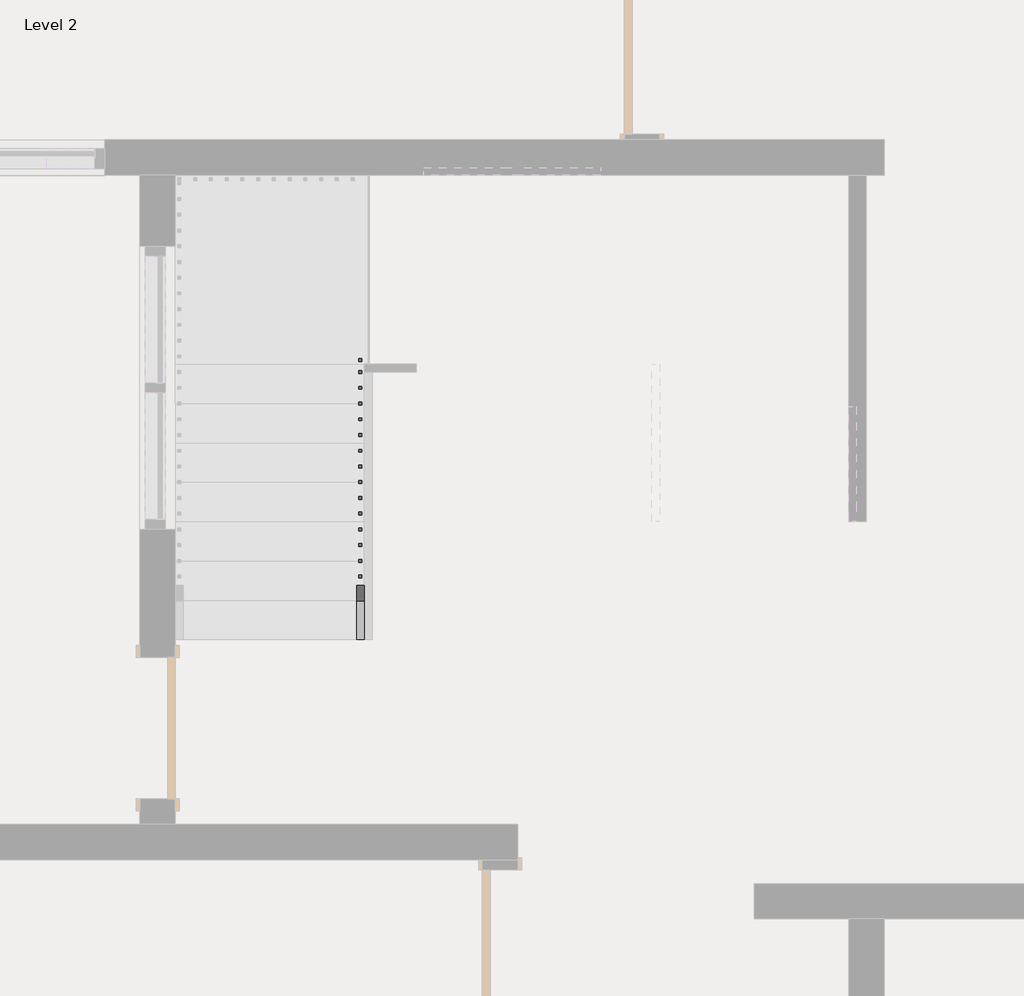
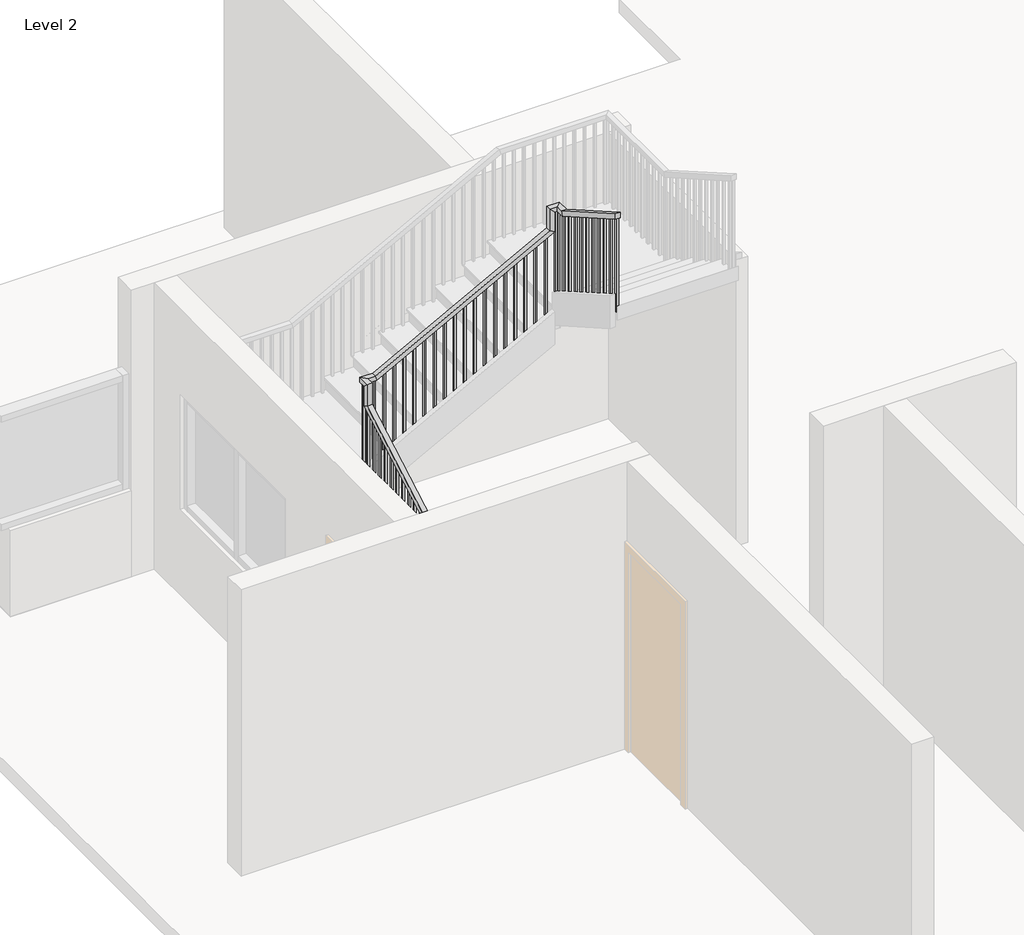
# One storey, part 4 of 5: 1 railing.
"""IFC4 building model written with IfcOpenShell, lengths in millimetres."""

from ifc_helpers import new_model, si_unit, frame, origin, place, context, project, spatial, polyline, outline, extrude, faceted_brep, element, save

model = new_model("IFC4")

# Units and contexts
model_context = context("Model", 3, world=origin())
ifc_project = project(units=[si_unit("LENGTHUNIT", "METRE", prefix="MILLI")], contexts=[model_context])

# Site, building, storey
site = spatial("IfcSite", under=ifc_project)
building = spatial("IfcBuilding", under=site)
storey = spatial("IfcBuildingStorey", under=building, Name="Level 2", Elevation=3048.0)

# Railing
placement = place(None, origin())
element("IfcRailing", 1, ObjectType="Handrail - Rectangular", at=placement, inside=storey, context=model_context, shape_type="SolidModel", body=[
    faceted_brep([(-39833.3146233, 12459.3864709, 4107.5428571), (-39833.3146233, 12459.3864709, 4049.0339009), (-39782.5146233, 12459.3864709, 4049.0339009), (-39782.5146233, 12459.3864709, 4107.5428571), (-39833.3146233, 14161.1864709, 5080.0), (-39833.3146233, 14211.9864709, 5050.5196152), (-39782.5146233, 14211.9864709, 5050.5196152), (-39782.5146233, 14161.1864709, 5080.0), (-39833.3146233, 14161.1864709, 5309.3257143), (-39833.3146233, 14211.9864709, 5258.5257143), (-39782.5146233, 14211.9864709, 5258.5257143), (-39782.5146233, 14161.1864709, 5309.3257143), (-39833.3146233, 14288.1864709, 5309.3257143), (-39833.3146233, 14288.1864709, 5258.5257143), (-39782.5146233, 14237.3864709, 5258.5257143), (-39782.5146233, 14237.3864709, 5309.3257143), (-39706.3146233, 14288.1864709, 5309.3257143), (-39693.6146233, 14288.1864709, 5258.5257143), (-39693.6146233, 14237.3864709, 5258.5257143), (-39706.3146233, 14237.3864709, 5309.3257143), (-37953.7146233, 14288.1864709, 6244.0457143), (-37902.9146233, 14288.1864709, 6213.5657143), (-37902.9146233, 14237.3864709, 6213.5657143), (-37953.7146233, 14237.3864709, 6244.0457143), (-37953.7146233, 14288.1864709, 6473.3714286), (-37902.9146233, 14288.1864709, 6422.5714286), (-37902.9146233, 14237.3864709, 6422.5714286), (-37953.7146233, 14237.3864709, 6473.3714286), (-37826.7146233, 14288.1864709, 6473.3714286), (-37826.7146233, 14288.1864709, 6422.5714286), (-37877.5146233, 14237.3864709, 6422.5714286), (-37877.5146233, 14237.3864709, 6473.3714286), (-37826.7146233, 14161.1864709, 6473.3714286), (-37826.7146233, 14147.6957975, 6422.5714286), (-37877.5146233, 14147.6957975, 6422.5714286), (-37877.5146233, 14161.1864709, 6473.3714286), (-37826.7146233, 13221.3864709, 7010.4), (-37877.5146233, 13221.3864709, 7010.4), (-37877.5146233, 13221.3864709, 6951.8910438), (-37826.7146233, 13221.3864709, 6951.8910438)], [[[0, 1, 2, 3]], [[1, 0, 4, 5]], [[2, 1, 5, 6]], [[3, 2, 6, 7]], [[0, 3, 7, 4]], [[5, 4, 8, 9]], [[6, 5, 9, 10]], [[7, 6, 10, 11]], [[4, 7, 11, 8]], [[9, 8, 12, 13]], [[10, 9, 13, 14]], [[11, 10, 14, 15]], [[8, 11, 15, 12]], [[13, 12, 16, 17]], [[14, 13, 17, 18]], [[15, 14, 18, 19]], [[12, 15, 19, 16]], [[17, 16, 20, 21]], [[18, 17, 21, 22]], [[19, 18, 22, 23]], [[16, 19, 23, 20]], [[21, 20, 24, 25]], [[22, 21, 25, 26]], [[23, 22, 26, 27]], [[20, 23, 27, 24]], [[25, 24, 28, 29]], [[26, 25, 29, 30]], [[27, 26, 30, 31]], [[24, 27, 31, 28]], [[29, 28, 32, 33]], [[30, 29, 33, 34]], [[31, 30, 34, 35]], [[28, 31, 35, 32]], [[36, 37, 38, 39]], [[33, 32, 36, 39]], [[34, 33, 39, 38]], [[35, 34, 38, 37]], [[32, 35, 37, 36]]]),
    extrude(outline(polyline([(13237.2614709, 6942.8196152), (13256.3114709, 6931.9339009), (13256.3114709, 5950.8571429), (13237.2614709, 5950.8571429), (13237.2614709, 6942.8196152)])), frame((-37861.6396233, 0.0, 0.0), z_axis=(1.0, 0.0, 0.0), x_axis=(0.0, 1.0, 0.0)), (0.0, 0.0, 1.0), 19.05),
    extrude(outline(polyline([(13338.8614709, 6884.7624723), (13357.9114709, 6873.8767581), (13357.9114709, 5950.8571429), (13338.8614709, 5950.8571429), (13338.8614709, 6884.7624723)])), frame((-37861.6396233, 0.0, 0.0), z_axis=(1.0, 0.0, 0.0), x_axis=(0.0, 1.0, 0.0)), (0.0, 0.0, 1.0), 19.05),
    extrude(outline(polyline([(13440.4614709, 6826.7053295), (13459.5114709, 6815.8196152), (13459.5114709, 5950.8571429), (13440.4614709, 5950.8571429), (13440.4614709, 6826.7053295)])), frame((-37861.6396233, 0.0, 0.0), z_axis=(1.0, 0.0, 0.0), x_axis=(0.0, 1.0, 0.0)), (0.0, 0.0, 1.0), 19.05),
    extrude(outline(polyline([(13542.0614709, 6768.6481866), (13561.1114709, 6757.7624723), (13561.1114709, 5805.7142857), (13542.0614709, 5805.7142857), (13542.0614709, 6768.6481866)])), frame((-37861.6396233, 0.0, 0.0), z_axis=(1.0, 0.0, 0.0), x_axis=(0.0, 1.0, 0.0)), (0.0, 0.0, 1.0), 19.05),
    extrude(outline(polyline([(13643.6614709, 6710.5910438), (13662.7114709, 6699.7053295), (13662.7114709, 5805.7142857), (13643.6614709, 5805.7142857), (13643.6614709, 6710.5910438)])), frame((-37861.6396233, 0.0, 0.0), z_axis=(1.0, 0.0, 0.0), x_axis=(0.0, 1.0, 0.0)), (0.0, 0.0, 1.0), 19.05),
    extrude(outline(polyline([(13745.2614709, 6652.5339009), (13764.3114709, 6641.6481866), (13764.3114709, 5660.5714286), (13745.2614709, 5660.5714286), (13745.2614709, 6652.5339009)])), frame((-37861.6396233, 0.0, 0.0), z_axis=(1.0, 0.0, 0.0), x_axis=(0.0, 1.0, 0.0)), (0.0, 0.0, 1.0), 19.05),
    extrude(outline(polyline([(13846.8614709, 6594.4767581), (13865.9114709, 6583.5910438), (13865.9114709, 5660.5714286), (13846.8614709, 5660.5714286), (13846.8614709, 6594.4767581)])), frame((-37861.6396233, 0.0, 0.0), z_axis=(1.0, 0.0, 0.0), x_axis=(0.0, 1.0, 0.0)), (0.0, 0.0, 1.0), 19.05),
    extrude(outline(polyline([(13948.4614709, 6536.4196152), (13967.5114709, 6525.5339009), (13967.5114709, 5660.5714286), (13948.4614709, 5660.5714286), (13948.4614709, 6536.4196152)])), frame((-37861.6396233, 0.0, 0.0), z_axis=(1.0, 0.0, 0.0), x_axis=(0.0, 1.0, 0.0)), (0.0, 0.0, 1.0), 19.05),
    extrude(outline(polyline([(14050.0614709, 6478.3624723), (14069.1114709, 6467.4767581), (14069.1114709, 5515.4285714), (14050.0614709, 5515.4285714), (14050.0614709, 6478.3624723)])), frame((-37861.6396233, 0.0, 0.0), z_axis=(1.0, 0.0, 0.0), x_axis=(0.0, 1.0, 0.0)), (0.0, 0.0, 1.0), 19.05),
    extrude(outline(polyline([(14151.6614709, 6420.3053295), (14170.7114709, 6409.4196152), (14170.7114709, 5515.4285714), (14151.6614709, 5515.4285714), (14151.6614709, 6420.3053295)])), frame((-37861.6396233, 0.0, 0.0), z_axis=(1.0, 0.0, 0.0), x_axis=(0.0, 1.0, 0.0)), (0.0, 0.0, 1.0), 19.05),
    extrude(outline(polyline([(-37887.0396233, 14253.2614709), (-37887.0396233, 14272.3114709), (-37867.9896233, 14272.3114709), (-37867.9896233, 14253.2614709), (-37887.0396233, 14253.2614709)])), frame((0.0, 0.0, 5370.2857143), z_axis=(0.0, 0.0, 1.0), x_axis=(1.0, 0.0, 0.0)), (0.0, 0.0, 1.0), 1052.2857143),
    extrude(outline(polyline([(6178.0057143, -37969.5896233), (6167.8457143, -37988.6396233), (5225.1428571, -37988.6396233), (5225.1428571, -37969.5896233), (6178.0057143, -37969.5896233)])), frame((0.0, 14253.2614709, 0.0), z_axis=(0.0, 1.0, 0.0), x_axis=(0.0, 0.0, 1.0)), (0.0, 0.0, 1.0), 19.05),
    extrude(outline(polyline([(6123.8190476, -38071.1896233), (6113.6590476, -38090.2396233), (5225.1428571, -38090.2396233), (5225.1428571, -38071.1896233), (6123.8190476, -38071.1896233)])), frame((0.0, 14253.2614709, 0.0), z_axis=(0.0, 1.0, 0.0), x_axis=(0.0, 0.0, 1.0)), (0.0, 0.0, 1.0), 19.05),
    extrude(outline(polyline([(6069.632381, -38172.7896233), (6059.472381, -38191.8396233), (5080.0, -38191.8396233), (5080.0, -38172.7896233), (6069.632381, -38172.7896233)])), frame((0.0, 14253.2614709, 0.0), z_axis=(0.0, 1.0, 0.0), x_axis=(0.0, 0.0, 1.0)), (0.0, 0.0, 1.0), 19.05),
    extrude(outline(polyline([(6015.4457143, -38274.3896233), (6005.2857143, -38293.4396233), (5080.0, -38293.4396233), (5080.0, -38274.3896233), (6015.4457143, -38274.3896233)])), frame((0.0, 14253.2614709, 0.0), z_axis=(0.0, 1.0, 0.0), x_axis=(0.0, 0.0, 1.0)), (0.0, 0.0, 1.0), 19.05),
    extrude(outline(polyline([(5961.2590476, -38375.9896233), (5951.0990476, -38395.0396233), (5080.0, -38395.0396233), (5080.0, -38375.9896233), (5961.2590476, -38375.9896233)])), frame((0.0, 14253.2614709, 0.0), z_axis=(0.0, 1.0, 0.0), x_axis=(0.0, 0.0, 1.0)), (0.0, 0.0, 1.0), 19.05),
    extrude(outline(polyline([(5907.072381, -38477.5896233), (5896.912381, -38496.6396233), (4934.8571429, -38496.6396233), (4934.8571429, -38477.5896233), (5907.072381, -38477.5896233)])), frame((0.0, 14253.2614709, 0.0), z_axis=(0.0, 1.0, 0.0), x_axis=(0.0, 0.0, 1.0)), (0.0, 0.0, 1.0), 19.05),
    extrude(outline(polyline([(5852.8857143, -38579.1896233), (5842.7257143, -38598.2396233), (4934.8571429, -38598.2396233), (4934.8571429, -38579.1896233), (5852.8857143, -38579.1896233)])), frame((0.0, 14253.2614709, 0.0), z_axis=(0.0, 1.0, 0.0), x_axis=(0.0, 0.0, 1.0)), (0.0, 0.0, 1.0), 19.05),
    extrude(outline(polyline([(5798.6990476, -38680.7896233), (5788.5390476, -38699.8396233), (4934.8571429, -38699.8396233), (4934.8571429, -38680.7896233), (5798.6990476, -38680.7896233)])), frame((0.0, 14253.2614709, 0.0), z_axis=(0.0, 1.0, 0.0), x_axis=(0.0, 0.0, 1.0)), (0.0, 0.0, 1.0), 19.05),
    extrude(outline(polyline([(5744.512381, -38782.3896233), (5734.352381, -38801.4396233), (4789.7142857, -38801.4396233), (4789.7142857, -38782.3896233), (5744.512381, -38782.3896233)])), frame((0.0, 14253.2614709, 0.0), z_axis=(0.0, 1.0, 0.0), x_axis=(0.0, 0.0, 1.0)), (0.0, 0.0, 1.0), 19.05),
    extrude(outline(polyline([(5690.3257143, -38883.9896233), (5680.1657143, -38903.0396233), (4789.7142857, -38903.0396233), (4789.7142857, -38883.9896233), (5690.3257143, -38883.9896233)])), frame((0.0, 14253.2614709, 0.0), z_axis=(0.0, 1.0, 0.0), x_axis=(0.0, 0.0, 1.0)), (0.0, 0.0, 1.0), 19.05),
    extrude(outline(polyline([(5636.1390476, -38985.5896233), (5625.9790476, -39004.6396233), (4644.5714286, -39004.6396233), (4644.5714286, -38985.5896233), (5636.1390476, -38985.5896233)])), frame((0.0, 14253.2614709, 0.0), z_axis=(0.0, 1.0, 0.0), x_axis=(0.0, 0.0, 1.0)), (0.0, 0.0, 1.0), 19.05),
    extrude(outline(polyline([(5581.952381, -39087.1896233), (5571.792381, -39106.2396233), (4644.5714286, -39106.2396233), (4644.5714286, -39087.1896233), (5581.952381, -39087.1896233)])), frame((0.0, 14253.2614709, 0.0), z_axis=(0.0, 1.0, 0.0), x_axis=(0.0, 0.0, 1.0)), (0.0, 0.0, 1.0), 19.05),
    extrude(outline(polyline([(5527.7657143, -39188.7896233), (5517.6057143, -39207.8396233), (4644.5714286, -39207.8396233), (4644.5714286, -39188.7896233), (5527.7657143, -39188.7896233)])), frame((0.0, 14253.2614709, 0.0), z_axis=(0.0, 1.0, 0.0), x_axis=(0.0, 0.0, 1.0)), (0.0, 0.0, 1.0), 19.05),
    extrude(outline(polyline([(5473.5790476, -39290.3896233), (5463.4190476, -39309.4396233), (4499.4285714, -39309.4396233), (4499.4285714, -39290.3896233), (5473.5790476, -39290.3896233)])), frame((0.0, 14253.2614709, 0.0), z_axis=(0.0, 1.0, 0.0), x_axis=(0.0, 0.0, 1.0)), (0.0, 0.0, 1.0), 19.05),
    extrude(outline(polyline([(5419.392381, -39391.9896233), (5409.232381, -39411.0396233), (4499.4285714, -39411.0396233), (4499.4285714, -39391.9896233), (5419.392381, -39391.9896233)])), frame((0.0, 14253.2614709, 0.0), z_axis=(0.0, 1.0, 0.0), x_axis=(0.0, 0.0, 1.0)), (0.0, 0.0, 1.0), 19.05),
    extrude(outline(polyline([(5365.2057143, -39493.5896233), (5355.0457143, -39512.6396233), (4499.4285714, -39512.6396233), (4499.4285714, -39493.5896233), (5365.2057143, -39493.5896233)])), frame((0.0, 14253.2614709, 0.0), z_axis=(0.0, 1.0, 0.0), x_axis=(0.0, 0.0, 1.0)), (0.0, 0.0, 1.0), 19.05),
    extrude(outline(polyline([(5311.0190476, -39595.1896233), (5300.8590476, -39614.2396233), (4354.2857143, -39614.2396233), (4354.2857143, -39595.1896233), (5311.0190476, -39595.1896233)])), frame((0.0, 14253.2614709, 0.0), z_axis=(0.0, 1.0, 0.0), x_axis=(0.0, 0.0, 1.0)), (0.0, 0.0, 1.0), 19.05),
    extrude(outline(polyline([(5256.832381, -39696.7896233), (5246.672381, -39715.8396233), (4354.2857143, -39715.8396233), (4354.2857143, -39696.7896233), (5256.832381, -39696.7896233)])), frame((0.0, 14253.2614709, 0.0), z_axis=(0.0, 1.0, 0.0), x_axis=(0.0, 0.0, 1.0)), (0.0, 0.0, 1.0), 19.05),
    extrude(outline(polyline([(-39798.3896233, 14177.0614709), (-39817.4396233, 14177.0614709), (-39817.4396233, 14196.1114709), (-39798.3896233, 14196.1114709), (-39798.3896233, 14177.0614709)])), frame((0.0, 0.0, 4064.0), z_axis=(0.0, 0.0, 1.0), x_axis=(1.0, 0.0, 0.0)), (0.0, 0.0, 1.0), 1194.5257143),
    extrude(outline(polyline([(14075.4614709, 4972.5053295), (14094.5114709, 4983.3910438), (14094.5114709, 4064.0), (14075.4614709, 4064.0), (14075.4614709, 4972.5053295)])), frame((-39817.4396233, 0.0, 0.0), z_axis=(1.0, 0.0, 0.0), x_axis=(0.0, 1.0, 0.0)), (0.0, 0.0, 1.0), 19.05),
    extrude(outline(polyline([(13973.8614709, 4914.4481866), (13992.9114709, 4925.3339009), (13992.9114709, 4064.0), (13973.8614709, 4064.0), (13973.8614709, 4914.4481866)])), frame((-39817.4396233, 0.0, 0.0), z_axis=(1.0, 0.0, 0.0), x_axis=(0.0, 1.0, 0.0)), (0.0, 0.0, 1.0), 19.05),
    extrude(outline(polyline([(13872.2614709, 4856.3910438), (13891.3114709, 4867.2767581), (13891.3114709, 3918.8571429), (13872.2614709, 3918.8571429), (13872.2614709, 4856.3910438)])), frame((-39817.4396233, 0.0, 0.0), z_axis=(1.0, 0.0, 0.0), x_axis=(0.0, 1.0, 0.0)), (0.0, 0.0, 1.0), 19.05),
    extrude(outline(polyline([(13770.6614709, 4798.3339009), (13789.7114709, 4809.2196152), (13789.7114709, 3918.8571429), (13770.6614709, 3918.8571429), (13770.6614709, 4798.3339009)])), frame((-39817.4396233, 0.0, 0.0), z_axis=(1.0, 0.0, 0.0), x_axis=(0.0, 1.0, 0.0)), (0.0, 0.0, 1.0), 19.05),
    extrude(outline(polyline([(13669.0614709, 4740.2767581), (13688.1114709, 4751.1624723), (13688.1114709, 3773.7142857), (13669.0614709, 3773.7142857), (13669.0614709, 4740.2767581)])), frame((-39817.4396233, 0.0, 0.0), z_axis=(1.0, 0.0, 0.0), x_axis=(0.0, 1.0, 0.0)), (0.0, 0.0, 1.0), 19.05),
    extrude(outline(polyline([(13567.4614709, 4682.2196152), (13586.5114709, 4693.1053295), (13586.5114709, 3773.7142857), (13567.4614709, 3773.7142857), (13567.4614709, 4682.2196152)])), frame((-39817.4396233, 0.0, 0.0), z_axis=(1.0, 0.0, 0.0), x_axis=(0.0, 1.0, 0.0)), (0.0, 0.0, 1.0), 19.05),
    extrude(outline(polyline([(13465.8614709, 4624.1624723), (13484.9114709, 4635.0481866), (13484.9114709, 3773.7142857), (13465.8614709, 3773.7142857), (13465.8614709, 4624.1624723)])), frame((-39817.4396233, 0.0, 0.0), z_axis=(1.0, 0.0, 0.0), x_axis=(0.0, 1.0, 0.0)), (0.0, 0.0, 1.0), 19.05),
    extrude(outline(polyline([(13364.2614709, 4566.1053295), (13383.3114709, 4576.9910438), (13383.3114709, 3628.5714286), (13364.2614709, 3628.5714286), (13364.2614709, 4566.1053295)])), frame((-39817.4396233, 0.0, 0.0), z_axis=(1.0, 0.0, 0.0), x_axis=(0.0, 1.0, 0.0)), (0.0, 0.0, 1.0), 19.05),
    extrude(outline(polyline([(13262.6614709, 4508.0481866), (13281.7114709, 4518.9339009), (13281.7114709, 3628.5714286), (13262.6614709, 3628.5714286), (13262.6614709, 4508.0481866)])), frame((-39817.4396233, 0.0, 0.0), z_axis=(1.0, 0.0, 0.0), x_axis=(0.0, 1.0, 0.0)), (0.0, 0.0, 1.0), 19.05),
    extrude(outline(polyline([(13161.0614709, 4449.9910438), (13180.1114709, 4460.8767581), (13180.1114709, 3483.4285714), (13161.0614709, 3483.4285714), (13161.0614709, 4449.9910438)])), frame((-39817.4396233, 0.0, 0.0), z_axis=(1.0, 0.0, 0.0), x_axis=(0.0, 1.0, 0.0)), (0.0, 0.0, 1.0), 19.05),
    extrude(outline(polyline([(13059.4614709, 4391.9339009), (13078.5114709, 4402.8196152), (13078.5114709, 3483.4285714), (13059.4614709, 3483.4285714), (13059.4614709, 4391.9339009)])), frame((-39817.4396233, 0.0, 0.0), z_axis=(1.0, 0.0, 0.0), x_axis=(0.0, 1.0, 0.0)), (0.0, 0.0, 1.0), 19.05),
    extrude(outline(polyline([(12957.8614709, 4333.8767581), (12976.9114709, 4344.7624723), (12976.9114709, 3483.4285714), (12957.8614709, 3483.4285714), (12957.8614709, 4333.8767581)])), frame((-39817.4396233, 0.0, 0.0), z_axis=(1.0, 0.0, 0.0), x_axis=(0.0, 1.0, 0.0)), (0.0, 0.0, 1.0), 19.05),
    extrude(outline(polyline([(12856.2614709, 4275.8196152), (12875.3114709, 4286.7053295), (12875.3114709, 3338.2857143), (12856.2614709, 3338.2857143), (12856.2614709, 4275.8196152)])), frame((-39817.4396233, 0.0, 0.0), z_axis=(1.0, 0.0, 0.0), x_axis=(0.0, 1.0, 0.0)), (0.0, 0.0, 1.0), 19.05),
    extrude(outline(polyline([(12754.6614709, 4217.7624723), (12773.7114709, 4228.6481866), (12773.7114709, 3338.2857143), (12754.6614709, 3338.2857143), (12754.6614709, 4217.7624723)])), frame((-39817.4396233, 0.0, 0.0), z_axis=(1.0, 0.0, 0.0), x_axis=(0.0, 1.0, 0.0)), (0.0, 0.0, 1.0), 19.05),
    extrude(outline(polyline([(12653.0614709, 4159.7053295), (12672.1114709, 4170.5910438), (12672.1114709, 3193.1428571), (12653.0614709, 3193.1428571), (12653.0614709, 4159.7053295)])), frame((-39817.4396233, 0.0, 0.0), z_axis=(1.0, 0.0, 0.0), x_axis=(0.0, 1.0, 0.0)), (0.0, 0.0, 1.0), 19.05),
    extrude(outline(polyline([(12551.4614709, 4101.6481866), (12570.5114709, 4112.5339009), (12570.5114709, 3193.1428571), (12551.4614709, 3193.1428571), (12551.4614709, 4101.6481866)])), frame((-39817.4396233, 0.0, 0.0), z_axis=(1.0, 0.0, 0.0), x_axis=(0.0, 1.0, 0.0)), (0.0, 0.0, 1.0), 19.05),
    extrude(outline(polyline([(-37861.6396233, 14253.2614709), (-37861.6396233, 14272.3114709), (-37842.5896233, 14272.3114709), (-37842.5896233, 14253.2614709), (-37861.6396233, 14253.2614709)])), frame((0.0, 0.0, 5370.2857143), z_axis=(0.0, 0.0, 1.0), x_axis=(1.0, 0.0, 0.0)), (0.0, 0.0, 1.0), 1052.2857143),
    extrude(outline(polyline([(-39798.3896233, 14253.2614709), (-39817.4396233, 14253.2614709), (-39817.4396233, 14272.3114709), (-39798.3896233, 14272.3114709), (-39798.3896233, 14253.2614709)])), frame((0.0, 0.0, 4209.1428571), z_axis=(0.0, 0.0, 1.0), x_axis=(1.0, 0.0, 0.0)), (0.0, 0.0, 1.0), 1049.3828571),
    extrude(outline(polyline([(13221.3864709, 6951.8910438), (13240.4364709, 6941.0053295), (13240.4364709, 5950.8571429), (13221.3864709, 5950.8571429), (13221.3864709, 6951.8910438)])), frame((-37861.6396233, 0.0, 0.0), z_axis=(1.0, 0.0, 0.0), x_axis=(0.0, 1.0, 0.0)), (0.0, 0.0, 1.0), 19.05),
    extrude(outline(polyline([(12459.3864709, 4049.0339009), (12478.4364709, 4059.9196152), (12478.4364709, 3193.1428571), (12459.3864709, 3193.1428571), (12459.3864709, 4049.0339009)])), frame((-39817.4396233, 0.0, 0.0), z_axis=(1.0, 0.0, 0.0), x_axis=(0.0, 1.0, 0.0)), (0.0, 0.0, 1.0), 19.05),
])

save(model, "model.ifc")

# Revit data of these elements
# Type "Handrail - Rectangular"
#   Assembly Code = "C2010400"
#   built-in parameter 1008612 = 0.0416667 (stored number, unit not read)
#   built-in parameter 1008611 = 0.0416667 (stored number, unit not read)
#   built-in parameter 1008609 = 0.333333 (stored number, unit not read)
#   built-in parameter 1008604 = 0.166667 (stored number, unit not read)
#   built-in parameter 1008603 = 0.166667 (stored number, unit not read)
#   Railing Height = 3' - 0"
#   built-in parameter 1008630 = 2
#   built-in parameter 1008610 = 2
#   built-in parameter 1008618 = Baluster - Square : 3/4"
# Element 1 (IfcRailing, "Handrail - Rectangular")
#   Phase Created = New Construction
